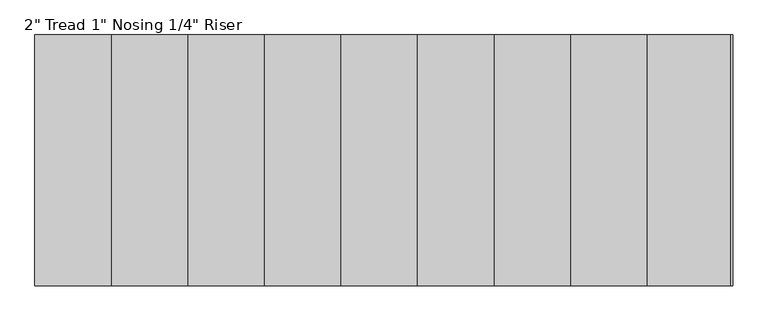
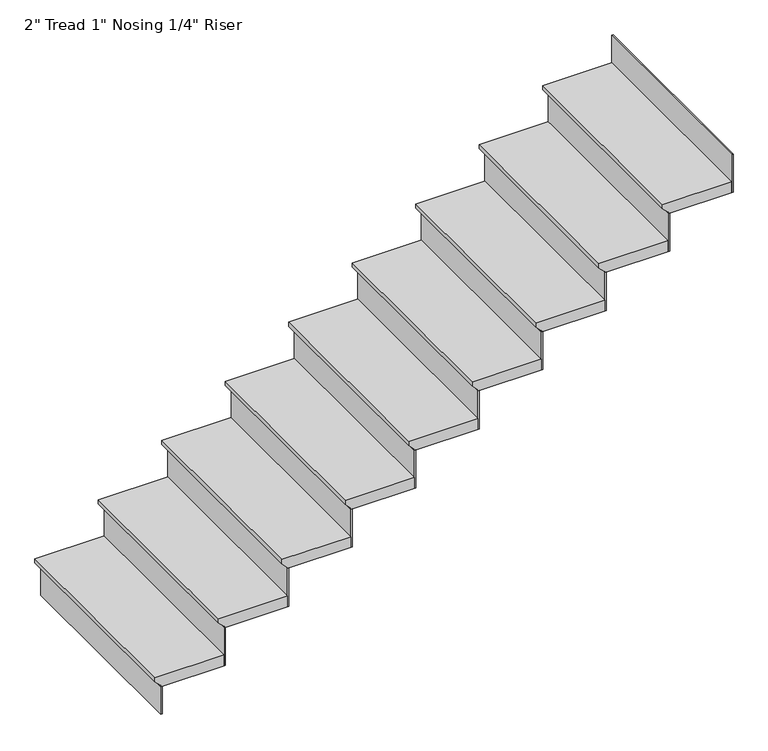
"""IFC4 building model written with IfcOpenShell, lengths in millimetres: stair flight geometry."""

from ifc_helpers import new_model, si_unit, origin, place, context, project, spatial, faceted_brep, source, transform, mapped, element, save


def stair_flight_cfa64765(model_context):
    return source(origin(), model_context, "Body", "Brep", [
        faceted_brep([(-4892.1918815, 2913.4168074, 768.35), (-4892.1918815, 2913.4168074, 787.4), (-4892.1918815, 3827.8168074, 787.4), (-4892.1918815, 3827.8168074, 768.35), (-4866.7918815, 2913.4168074, 742.95), (-4866.7918815, 3827.8168074, 742.95), (-4587.3918815, 2913.4168074, 787.4), (-4587.3918815, 3827.8168074, 787.4), (-4866.7918815, 3827.8168074, 736.6), (-4587.3918815, 3827.8168074, 736.6), (-4587.3918815, 2913.4168074, 736.6), (-4866.7918815, 2913.4168074, 736.6)], [[[0, 1, 2, 3]], [[4, 0, 3, 5]], [[2, 1, 6, 7]], [[8, 9, 10, 11]], [[2, 7, 9, 8, 5, 3]], [[8, 11, 4, 5]], [[6, 1, 0, 4, 11, 10]], [[7, 6, 10, 9]]]),
        faceted_brep([(-4866.7918815, 2913.4168074, 736.6), (-4866.7918815, 2913.4168074, 609.6), (-4860.4418815, 2913.4168074, 609.6), (-4860.4418815, 2913.4168074, 736.6), (-4866.7918815, 3827.8168074, 736.6), (-4860.4418815, 3827.8168074, 736.6), (-4860.4418815, 3827.8168074, 609.6), (-4866.7918815, 3827.8168074, 609.6)], [[[0, 1, 2, 3]], [[4, 5, 6, 7]], [[1, 0, 4, 7]], [[2, 1, 7, 6]], [[3, 2, 6, 5]], [[0, 3, 5, 4]]]),
        faceted_brep([(-4587.3918815, 2913.4168074, 914.4), (-4587.3918815, 2913.4168074, 736.6), (-4581.0418815, 2913.4168074, 736.6), (-4581.0418815, 2913.4168074, 914.4), (-4587.3918815, 3827.8168074, 914.4), (-4581.0418815, 3827.8168074, 914.4), (-4581.0418815, 3827.8168074, 736.6), (-4587.3918815, 3827.8168074, 736.6)], [[[0, 1, 2, 3]], [[4, 5, 6, 7]], [[1, 0, 4, 7]], [[2, 1, 7, 6]], [[3, 2, 6, 5]], [[0, 3, 5, 4]]]),
        faceted_brep([(-4612.7918815, 3827.8168074, 965.2), (-4612.7918815, 2913.4168074, 965.2), (-4307.9918815, 2913.4168074, 965.2), (-4307.9918815, 3827.8168074, 965.2), (-4587.3918815, 3827.8168074, 914.4), (-4307.9918815, 3827.8168074, 914.4), (-4307.9918815, 2913.4168074, 914.4), (-4587.3918815, 2913.4168074, 914.4), (-4587.3918815, 3827.8168074, 920.75), (-4612.7918815, 3827.8168074, 946.15), (-4587.3918815, 2913.4168074, 920.75), (-4612.7918815, 2913.4168074, 946.15)], [[[0, 1, 2, 3]], [[4, 5, 6, 7]], [[0, 3, 5, 4, 8, 9]], [[4, 7, 10, 8]], [[2, 1, 11, 10, 7, 6]], [[3, 2, 6, 5]], [[11, 1, 0, 9]], [[10, 11, 9, 8]]]),
        faceted_brep([(-4307.9918815, 2913.4168074, 1092.2), (-4307.9918815, 2913.4168074, 914.4), (-4301.6418815, 2913.4168074, 914.4), (-4301.6418815, 2913.4168074, 1092.2), (-4307.9918815, 3827.8168074, 1092.2), (-4301.6418815, 3827.8168074, 1092.2), (-4301.6418815, 3827.8168074, 914.4), (-4307.9918815, 3827.8168074, 914.4)], [[[0, 1, 2, 3]], [[4, 5, 6, 7]], [[1, 0, 4, 7]], [[2, 1, 7, 6]], [[3, 2, 6, 5]], [[0, 3, 5, 4]]]),
        faceted_brep([(-4333.3918815, 3827.8168074, 1143.0), (-4333.3918815, 2913.4168074, 1143.0), (-4028.5918815, 2913.4168074, 1143.0), (-4028.5918815, 3827.8168074, 1143.0), (-4307.9918815, 3827.8168074, 1092.2), (-4028.5918815, 3827.8168074, 1092.2), (-4028.5918815, 2913.4168074, 1092.2), (-4307.9918815, 2913.4168074, 1092.2), (-4307.9918815, 3827.8168074, 1098.55), (-4333.3918815, 3827.8168074, 1123.95), (-4307.9918815, 2913.4168074, 1098.55), (-4333.3918815, 2913.4168074, 1123.95)], [[[0, 1, 2, 3]], [[4, 5, 6, 7]], [[0, 3, 5, 4, 8, 9]], [[4, 7, 10, 8]], [[2, 1, 11, 10, 7, 6]], [[3, 2, 6, 5]], [[11, 1, 0, 9]], [[10, 11, 9, 8]]]),
        faceted_brep([(-4028.5918815, 2913.4168074, 1270.0), (-4028.5918815, 2913.4168074, 1092.2), (-4022.2418815, 2913.4168074, 1092.2), (-4022.2418815, 2913.4168074, 1270.0), (-4028.5918815, 3827.8168074, 1270.0), (-4022.2418815, 3827.8168074, 1270.0), (-4022.2418815, 3827.8168074, 1092.2), (-4028.5918815, 3827.8168074, 1092.2)], [[[0, 1, 2, 3]], [[4, 5, 6, 7]], [[1, 0, 4, 7]], [[2, 1, 7, 6]], [[3, 2, 6, 5]], [[0, 3, 5, 4]]]),
        faceted_brep([(-4053.9918815, 3827.8168074, 1320.8), (-4053.9918815, 2913.4168074, 1320.8), (-3749.1918815, 2913.4168074, 1320.8), (-3749.1918815, 3827.8168074, 1320.8), (-4028.5918815, 3827.8168074, 1270.0), (-3749.1918815, 3827.8168074, 1270.0), (-3749.1918815, 2913.4168074, 1270.0), (-4028.5918815, 2913.4168074, 1270.0), (-4028.5918815, 3827.8168074, 1276.35), (-4053.9918815, 3827.8168074, 1301.75), (-4028.5918815, 2913.4168074, 1276.35), (-4053.9918815, 2913.4168074, 1301.75)], [[[0, 1, 2, 3]], [[4, 5, 6, 7]], [[0, 3, 5, 4, 8, 9]], [[4, 7, 10, 8]], [[2, 1, 11, 10, 7, 6]], [[3, 2, 6, 5]], [[11, 1, 0, 9]], [[10, 11, 9, 8]]]),
        faceted_brep([(-3749.1918815, 2913.4168074, 1447.8), (-3749.1918815, 2913.4168074, 1270.0), (-3742.8418815, 2913.4168074, 1270.0), (-3742.8418815, 2913.4168074, 1447.8), (-3749.1918815, 3827.8168074, 1447.8), (-3742.8418815, 3827.8168074, 1447.8), (-3742.8418815, 3827.8168074, 1270.0), (-3749.1918815, 3827.8168074, 1270.0)], [[[0, 1, 2, 3]], [[4, 5, 6, 7]], [[1, 0, 4, 7]], [[2, 1, 7, 6]], [[3, 2, 6, 5]], [[0, 3, 5, 4]]]),
        faceted_brep([(-3774.5918815, 3827.8168074, 1498.6), (-3774.5918815, 2913.4168074, 1498.6), (-3469.7918815, 2913.4168074, 1498.6), (-3469.7918815, 3827.8168074, 1498.6), (-3749.1918815, 3827.8168074, 1447.8), (-3469.7918815, 3827.8168074, 1447.8), (-3469.7918815, 2913.4168074, 1447.8), (-3749.1918815, 2913.4168074, 1447.8), (-3749.1918815, 3827.8168074, 1454.15), (-3774.5918815, 3827.8168074, 1479.55), (-3749.1918815, 2913.4168074, 1454.15), (-3774.5918815, 2913.4168074, 1479.55)], [[[0, 1, 2, 3]], [[4, 5, 6, 7]], [[0, 3, 5, 4, 8, 9]], [[4, 7, 10, 8]], [[2, 1, 11, 10, 7, 6]], [[3, 2, 6, 5]], [[11, 1, 0, 9]], [[10, 11, 9, 8]]]),
        faceted_brep([(-3469.7918815, 2913.4168074, 1625.6), (-3469.7918815, 2913.4168074, 1447.8), (-3463.4418815, 2913.4168074, 1447.8), (-3463.4418815, 2913.4168074, 1625.6), (-3469.7918815, 3827.8168074, 1625.6), (-3463.4418815, 3827.8168074, 1625.6), (-3463.4418815, 3827.8168074, 1447.8), (-3469.7918815, 3827.8168074, 1447.8)], [[[0, 1, 2, 3]], [[4, 5, 6, 7]], [[1, 0, 4, 7]], [[2, 1, 7, 6]], [[3, 2, 6, 5]], [[0, 3, 5, 4]]]),
        faceted_brep([(-3495.1918815, 3827.8168074, 1676.4), (-3495.1918815, 2913.4168074, 1676.4), (-3190.3918815, 2913.4168074, 1676.4), (-3190.3918815, 3827.8168074, 1676.4), (-3469.7918815, 3827.8168074, 1625.6), (-3190.3918815, 3827.8168074, 1625.6), (-3190.3918815, 2913.4168074, 1625.6), (-3469.7918815, 2913.4168074, 1625.6), (-3469.7918815, 3827.8168074, 1631.95), (-3495.1918815, 3827.8168074, 1657.35), (-3469.7918815, 2913.4168074, 1631.95), (-3495.1918815, 2913.4168074, 1657.35)], [[[0, 1, 2, 3]], [[4, 5, 6, 7]], [[0, 3, 5, 4, 8, 9]], [[4, 7, 10, 8]], [[2, 1, 11, 10, 7, 6]], [[3, 2, 6, 5]], [[11, 1, 0, 9]], [[10, 11, 9, 8]]]),
        faceted_brep([(-3190.3918815, 2913.4168074, 1803.4), (-3190.3918815, 2913.4168074, 1625.6), (-3184.0418815, 2913.4168074, 1625.6), (-3184.0418815, 2913.4168074, 1803.4), (-3190.3918815, 3827.8168074, 1803.4), (-3184.0418815, 3827.8168074, 1803.4), (-3184.0418815, 3827.8168074, 1625.6), (-3190.3918815, 3827.8168074, 1625.6)], [[[0, 1, 2, 3]], [[4, 5, 6, 7]], [[1, 0, 4, 7]], [[2, 1, 7, 6]], [[3, 2, 6, 5]], [[0, 3, 5, 4]]]),
        faceted_brep([(-3215.7918815, 3827.8168074, 1854.2), (-3215.7918815, 2913.4168074, 1854.2), (-2910.9918815, 2913.4168074, 1854.2), (-2910.9918815, 3827.8168074, 1854.2), (-3190.3918815, 3827.8168074, 1803.4), (-2910.9918815, 3827.8168074, 1803.4), (-2910.9918815, 2913.4168074, 1803.4), (-3190.3918815, 2913.4168074, 1803.4), (-3190.3918815, 3827.8168074, 1809.75), (-3215.7918815, 3827.8168074, 1835.15), (-3190.3918815, 2913.4168074, 1809.75), (-3215.7918815, 2913.4168074, 1835.15)], [[[0, 1, 2, 3]], [[4, 5, 6, 7]], [[0, 3, 5, 4, 8, 9]], [[4, 7, 10, 8]], [[2, 1, 11, 10, 7, 6]], [[3, 2, 6, 5]], [[11, 1, 0, 9]], [[10, 11, 9, 8]]]),
        faceted_brep([(-2910.9918815, 2913.4168074, 1981.2), (-2910.9918815, 2913.4168074, 1803.4), (-2904.6418815, 2913.4168074, 1803.4), (-2904.6418815, 2913.4168074, 1981.2), (-2910.9918815, 3827.8168074, 1981.2), (-2904.6418815, 3827.8168074, 1981.2), (-2904.6418815, 3827.8168074, 1803.4), (-2910.9918815, 3827.8168074, 1803.4)], [[[0, 1, 2, 3]], [[4, 5, 6, 7]], [[1, 0, 4, 7]], [[2, 1, 7, 6]], [[3, 2, 6, 5]], [[0, 3, 5, 4]]]),
        faceted_brep([(-2936.3918815, 3827.8168074, 2032.0), (-2936.3918815, 2913.4168074, 2032.0), (-2631.5918815, 2913.4168074, 2032.0), (-2631.5918815, 3827.8168074, 2032.0), (-2910.9918815, 3827.8168074, 1981.2), (-2631.5918815, 3827.8168074, 1981.2), (-2631.5918815, 2913.4168074, 1981.2), (-2910.9918815, 2913.4168074, 1981.2), (-2910.9918815, 3827.8168074, 1987.55), (-2936.3918815, 3827.8168074, 2012.95), (-2910.9918815, 2913.4168074, 1987.55), (-2936.3918815, 2913.4168074, 2012.95)], [[[0, 1, 2, 3]], [[4, 5, 6, 7]], [[0, 3, 5, 4, 8, 9]], [[4, 7, 10, 8]], [[2, 1, 11, 10, 7, 6]], [[3, 2, 6, 5]], [[11, 1, 0, 9]], [[10, 11, 9, 8]]]),
        faceted_brep([(-2352.1918815, 2913.4168074, 2336.8), (-2352.1918815, 2913.4168074, 2159.0), (-2345.8418815, 2913.4168074, 2159.0), (-2345.8418815, 2913.4168074, 2336.8), (-2352.1918815, 3827.8168074, 2336.8), (-2345.8418815, 3827.8168074, 2336.8), (-2345.8418815, 3827.8168074, 2159.0), (-2352.1918815, 3827.8168074, 2159.0)], [[[0, 1, 2, 3]], [[4, 5, 6, 7]], [[1, 0, 4, 7]], [[2, 1, 7, 6]], [[3, 2, 6, 5]], [[0, 3, 5, 4]]]),
        faceted_brep([(-2631.5918815, 2913.4168074, 2159.0), (-2631.5918815, 2913.4168074, 1981.2), (-2625.2418815, 2913.4168074, 1981.2), (-2625.2418815, 2913.4168074, 2159.0), (-2631.5918815, 3827.8168074, 2159.0), (-2625.2418815, 3827.8168074, 2159.0), (-2625.2418815, 3827.8168074, 1981.2), (-2631.5918815, 3827.8168074, 1981.2)], [[[0, 1, 2, 3]], [[4, 5, 6, 7]], [[1, 0, 4, 7]], [[2, 1, 7, 6]], [[3, 2, 6, 5]], [[0, 3, 5, 4]]]),
        faceted_brep([(-2352.1918815, 3827.8168074, 2209.8), (-2377.5918815, 3827.8168074, 2209.8), (-2656.9918815, 3827.8168074, 2209.8), (-2656.9918815, 2913.4168074, 2209.8), (-2352.1918815, 2913.4168074, 2209.8), (-2377.5918815, 3827.8168074, 2159.0), (-2352.1918815, 3827.8168074, 2159.0), (-2352.1918815, 2913.4168074, 2159.0), (-2631.5918815, 2913.4168074, 2159.0), (-2631.5918815, 3827.8168074, 2159.0), (-2631.5918815, 3827.8168074, 2165.35), (-2656.9918815, 3827.8168074, 2190.75), (-2631.5918815, 2913.4168074, 2165.35), (-2656.9918815, 2913.4168074, 2190.75)], [[[0, 1, 2, 3, 4]], [[5, 6, 7, 8, 9]], [[1, 0, 6, 5]], [[2, 1, 5, 9, 10, 11]], [[9, 8, 12, 10]], [[4, 3, 13, 12, 8, 7]], [[0, 4, 7, 6]], [[13, 3, 2, 11]], [[12, 13, 11, 10]]]),
    ])


if __name__ == "__main__":
    model = new_model("IFC4")
    model_context = context("Model", 3, world=origin())
    ifc_project = project(units=[si_unit("LENGTHUNIT", "METRE", prefix="MILLI")], contexts=[model_context])
    site = spatial("IfcSite", under=ifc_project)
    building = spatial("IfcBuilding", under=site)
    placement = place(None, origin())
    stair_flight_shape = stair_flight_cfa64765(model_context)
    element("IfcStairFlight", 1, ObjectType="2\" Tread 1\" Nosing 1/4\" Riser", at=placement, inside=building, context=model_context, shape_type="MappedRepresentation", body=[
        mapped(stair_flight_shape, transform((0.0, 0.0, 0.0), x_axis=(1.0, 0.0, 0.0), y_axis=(0.0, 1.0, 0.0), z_axis=(0.0, 0.0, 1.0))),
    ])
    save(model, "model.ifc")
